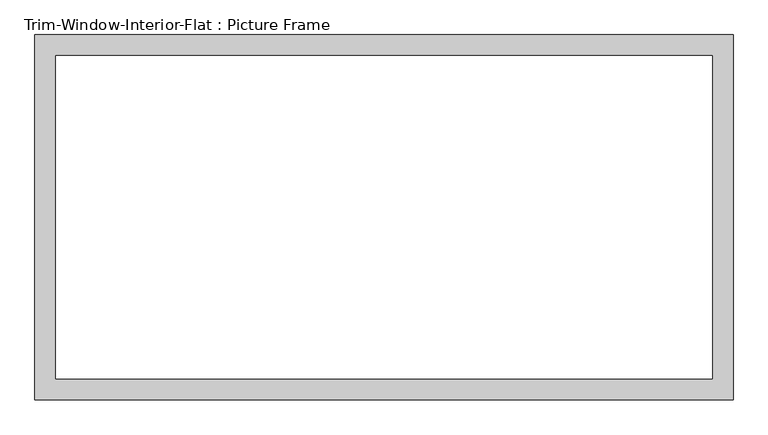
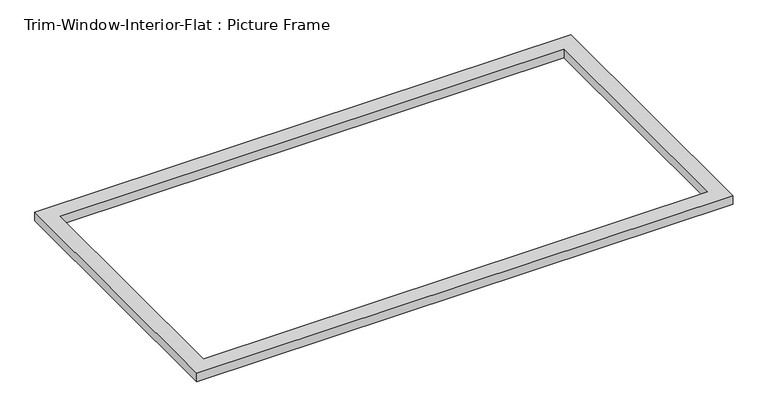
"""IFC4 building model written with IfcOpenShell, lengths in millimetres: proxy geometry, Trim-Window-Interior-Flat : Picture Frame."""

from ifc_helpers import new_model, si_unit, origin, origin_with_axes, place, context, project, spatial, polyline, outline, extrude, source, transform, mapped, element, save


def trim_window_interior_flat_picture_frame_0edfbaa2(model_context):
    return source(origin(), model_context, "Body", "SweptSolid", [
        extrude(outline(polyline([(958.85, 44.45), (958.85, -958.85), (-958.85, -958.85), (-958.85, 44.45), (958.85, 44.45)]), holes=[polyline([(901.7, -12.7), (-901.7, -12.7), (-901.7, -901.7), (901.7, -901.7), (901.7, -12.7)])]), origin_with_axes(), (0.0, 0.0, 1.0), 31.75),
    ])


if __name__ == "__main__":
    model = new_model("IFC4")
    model_context = context("Model", 3, world=origin())
    ifc_project = project(units=[si_unit("LENGTHUNIT", "METRE", prefix="MILLI")], contexts=[model_context])
    site = spatial("IfcSite", under=ifc_project)
    building = spatial("IfcBuilding", under=site)
    placement = place(None, origin())
    trim_window_interior_flat_picture_frame_shape = trim_window_interior_flat_picture_frame_0edfbaa2(model_context)
    element("IfcBuildingElementProxy", 1, Name="Trim-Window-Interior-Flat : Picture Frame", ObjectType="Trim-Window-Interior-Flat : Picture Frame", at=placement, inside=building, context=model_context, shape_type="MappedRepresentation", body=[
        mapped(trim_window_interior_flat_picture_frame_shape, transform((0.0, 0.0, 0.0), x_axis=(1.0, 0.0, 0.0), y_axis=(0.0, 1.0, 0.0), z_axis=(0.0, 0.0, 1.0))),
    ])
    save(model, "model.ifc")

# Revit data of these elements
# Type "Trim-Window-Interior-Flat : Picture Frame"
#   Trim Thickness_Picture Frame = 0' - 1 1/4"
#   Trim Width = 0' - 2 1/4"
#   Trim Thickness_with Sill = 0' - 0 3/4"
#   Sill Thickness = 0' - 1 1/4"
#   Opening Width [instance default] = 2' - 0"
#   Opening Height [instance default] = 3' - 0"
#   Default Elevation = 4' - 0"
#   Sill = no
#   Picture Frame = yes
#   Trim Material [instance default] = none
# Element 1 (IfcBuildingElementProxy, "Trim-Window-Interior-Flat : Picture Frame")
#   Opening Width = 6' - 0"
#   Trim Material = Wood - Stained
#   Materials on its faces: "Wood - Stained"
# Materials
#   "Wood - Stained": class "Wood", colour RGB 224 178 126, transparency 0, Cost = 0
